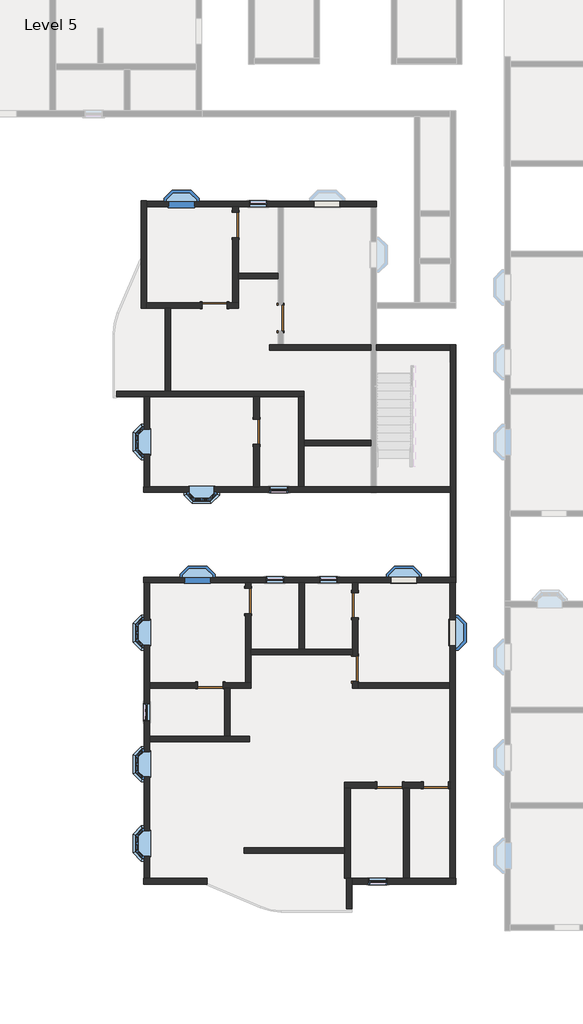
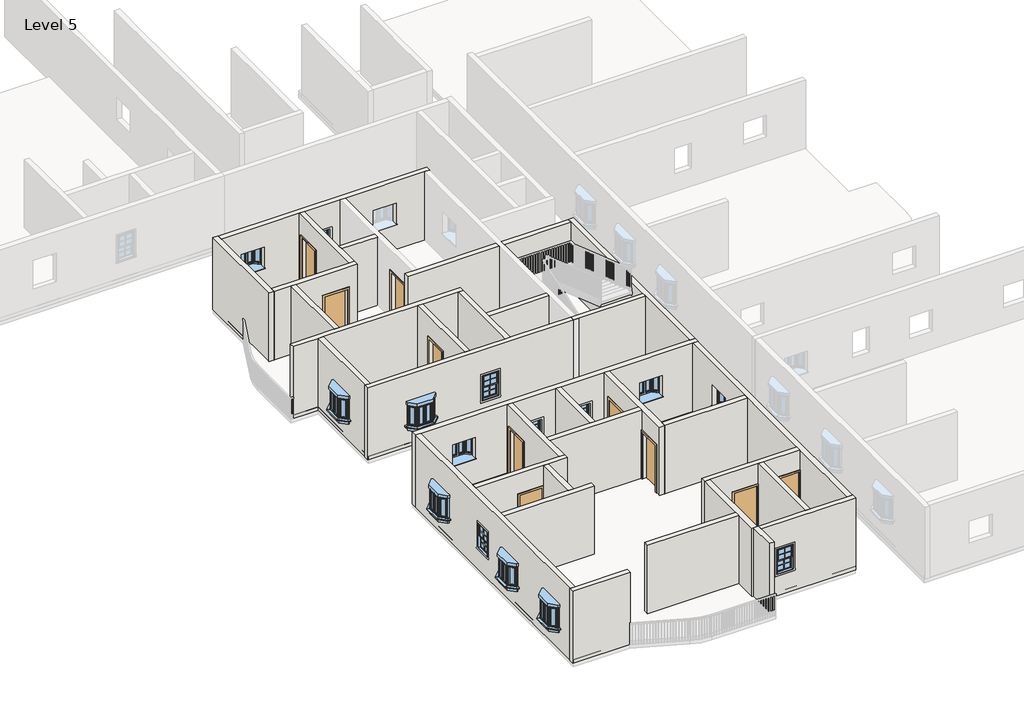
# One storey, part 1 of 14: 32 walls, 15 windows, 10 doors.
# Revit data of these elements (continued)
# Element 54 (IfcWindow, "Window-Double-Hung : 26\" x 42\"") (continued)
#   Window Inset = 0' - 0"
#   Interior Wall Closure = 0' - 1 1/2"
#   Frame Extension = 0' - 1 1/4"
#   Exterior Wall Closure = 0' - 0 1/2"
#   Interior Trim Visibility = yes
#   Indicator Visibility = yes
#   Exterior Trim Visibility = yes
#   Phase Created = New Construction
#   Materials on its faces: "Wood - Stained", "Glass", "Clad - White"
# Element 55 (IfcWindow, "Window-Double-Hung : 26\" x 42\"")
#   Mark = "269"
#   Window Inset = 0' - 0"
#   Interior Wall Closure = 0' - 1 1/2"
#   Frame Extension = 0' - 1 1/4"
#   Exterior Wall Closure = 0' - 0 1/2"
#   Interior Trim Visibility = yes
#   Indicator Visibility = yes
#   Exterior Trim Visibility = yes
#   Phase Created = New Construction
#   Materials on its faces: "Wood - Stained", "Glass", "Clad - White"
# Element 56 (IfcWindow, "Window-Double-Hung : 26\" x 42\"")
#   Mark = "270"
#   Window Inset = 0' - 0"
#   Interior Wall Closure = 0' - 1 1/2"
#   Frame Extension = 0' - 1 1/4"
#   Exterior Wall Closure = 0' - 0 1/2"
#   Interior Trim Visibility = yes
#   Indicator Visibility = yes
#   Exterior Trim Visibility = yes
#   Phase Created = New Construction
#   Materials on its faces: "Wood - Stained", "Glass", "Clad - White"
# Element 57 (IfcWindow, "Window-Double-Hung : 26\" x 42\"")
#   Mark = "271"
#   Window Inset = 0' - 0"
#   Interior Wall Closure = 0' - 1 1/2"
#   Frame Extension = 0' - 1 1/4"
#   Exterior Wall Closure = 0' - 0 1/2"
#   Interior Trim Visibility = yes
#   Indicator Visibility = yes
#   Exterior Trim Visibility = yes
#   Phase Created = New Construction
#   Materials on its faces: "Wood - Stained", "Glass", "Clad - White"
# Materials
#   "Door - Panel": class "Wood", colour RGB 210 159 95, transparency 0, Cost = 0
#   "Door - Frame": colour RGB 118 70 51, transparency 0, Cost = 0
#   "Window Frame": colour RGB 249 249 249, transparency 0
#   "Glass": class "Glass", colour RGB 0 128 192, transparency 0.75, Description = "Soda Lime Glass", Cost = 0
#   "Wood - Stained": class "Wood", colour RGB 224 178 126, transparency 0, Cost = 0
#   "Clad - White": class "Wood", colour RGB 242 242 238, transparency 0, Cost = 0
#   "Default Wall": colour RGB 128 128 128, transparency 0, Cost = 0
#   "Earth": class "Generic", colour RGB 97 75 62, transparency 0, Description = "Soil", Cost = 0
#   "Parking Stripe": class "Paint", colour RGB 250 250 91, transparency 0, Cost = 0
#   "Carpet (1)": class "Carpet", colour RGB 124 80 67, transparency 0, Description = "Interior finish", Cost = 0
#   "Softwood, Lumber": class "Wood", colour RGB 223 192 134, transparency 0, Description = "Pinus Echinata", Cost = 0
